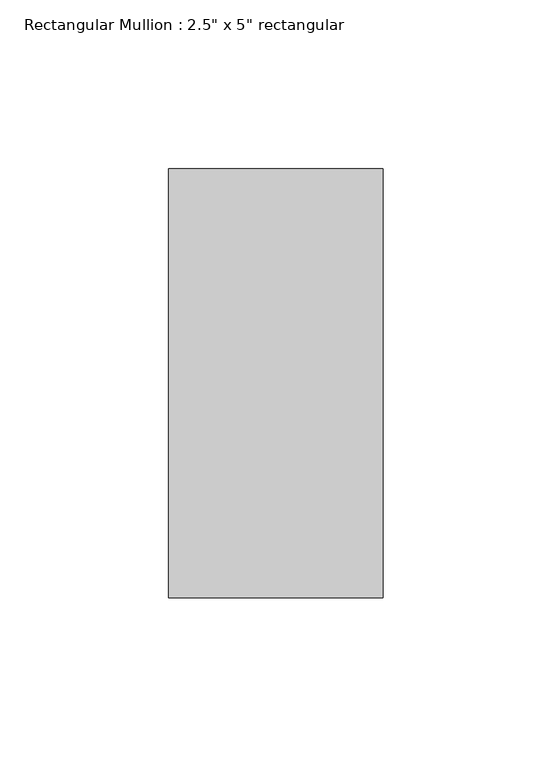
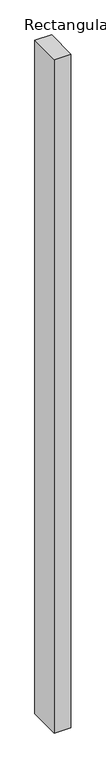
"""IFC4 building model written with IfcOpenShell, lengths in millimetres: member geometry."""

from ifc_helpers import new_model, si_unit, frame, origin, place, context, project, spatial, polyline, outline, extrude, source, transform, mapped, element, save


def member_25b70949(model_context):
    return source(origin(), model_context, "Body", "SweptSolid", [
        extrude(outline(polyline([(0.0, 63.5), (0.0, -63.5), (-63.5, -63.5), (-63.5, 63.5), (0.0, 63.5)])), frame((0.0, 0.0, -2704.8948327), z_axis=(0.0, 0.0, 1.0), x_axis=(1.0, 0.0, 0.0)), (0.0, 0.0, 1.0), 2704.8948327),
    ])


if __name__ == "__main__":
    model = new_model("IFC4")
    model_context = context("Model", 3, world=origin())
    ifc_project = project(units=[si_unit("LENGTHUNIT", "METRE", prefix="MILLI")], contexts=[model_context])
    site = spatial("IfcSite", under=ifc_project)
    building = spatial("IfcBuilding", under=site)
    placement = place(None, origin())
    member_shape = member_25b70949(model_context)
    element("IfcMember", 1, ObjectType="Rectangular Mullion : 2.5\" x 5\" rectangular", at=placement, inside=building, context=model_context, shape_type="MappedRepresentation", body=[
        mapped(member_shape, transform((0.0, 0.0, 0.0), x_axis=(1.0, 0.0, 0.0), y_axis=(0.0, 1.0, 0.0), z_axis=(0.0, 0.0, 1.0))),
    ])
    save(model, "model.ifc")

# Revit data of these elements
# Type "Rectangular Mullion : 2.5\" x 5\" rectangular"
#   built-in parameter 1007304 = 0.416667 (stored number, unit not read)
#   built-in parameter 1007301 = 0.104167 (stored number, unit not read)
#   built-in parameter 1007300 = 0.104167 (stored number, unit not read)
# Element 1 (IfcMember, "Rectangular Mullion : 2.5\" x 5\" rectangular")
#   Materials on its faces: "Damp-proofing"
# Materials
#   "Damp-proofing": class "Generic", colour RGB 127 127 127, transparency 0, Description = "Damp-proofing", Cost = 0
